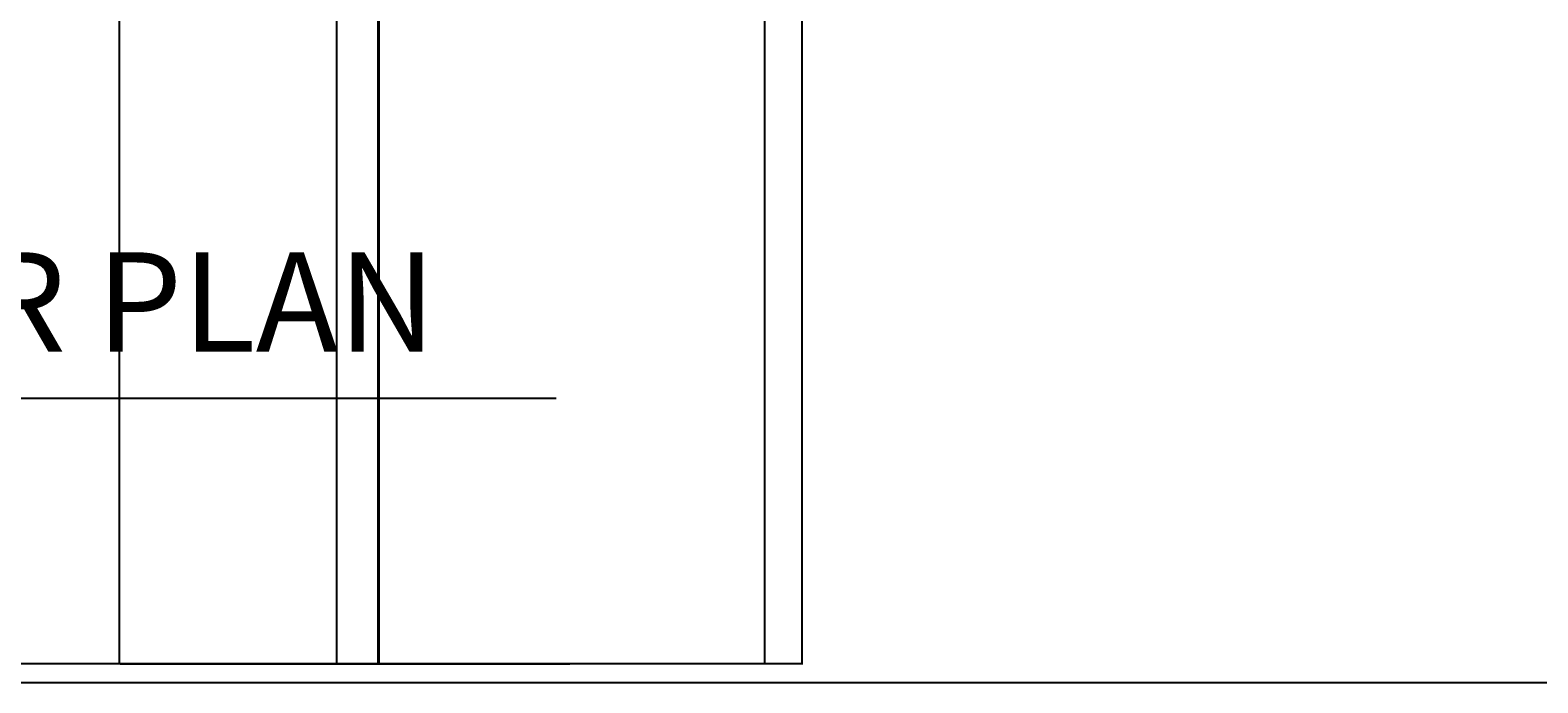
# Model space of a CAD drawing. Units: inches. Extents: x 1770 to 2988, y 1161 to 3221.
# Tile 2 of 44: x 2439 to 2804, y 1161 to 1319. Entities that reach past the tile are written whole.
import ezdxf

# ---------------------------------------------------------------- set-up
doc = ezdxf.new("R2010")
doc.units = ezdxf.units.IN
for name, color, linetype, lineweight in [('A-ANNO-DIMS', 2, 'Continuous', 18), ('A-ANNO-TEXT', 7, 'Continuous', 25), ('A-ANNO-TTLB', 7, 'Continuous', 25)]:
    doc.layers.add(name, color=color, linetype=linetype, lineweight=lineweight)
doc.styles.get("Standard").update_dxf_attribs({"font": 'arial.ttf'})
doc.dimstyles.get("Standard").update_dxf_attribs({"dimtxt": 0.18, "dimasz": 0.18, "dimexe": 0.18, "dimexo": 0.0625, "dimgap": 0.09, "dimtad": 0, "dimtih": 1, "dimtoh": 1, "dimdec": 4, "dimzin": 0, "dimdsep": 46, "dimtxsty": 'Standard', "dimcen": 0.09, "dimadec": 0, "dimazin": 0, "dimtfac": 1, "dimtdec": 4, "dimtofl": 0, "dimtmove": 0, "dimatfit": 3, "dimfxl": 1, "dimtolj": 1, "dimtzin": 0, "dimarcsym": 0})

# ---------------------------------------------------------------- blocks, each defined once
blk = doc.blocks.new('*D60')
at = {"layer": 'A-ANNO-DIMS', "color": 0, "lineweight": -2, "transparency": 16777216}
for p, q in [((2151.7, 1610.14), (2151.7, 1165.57)), ((2625.7, 1610.14), (2625.7, 1165.57)), ((2151.88, 1165.75), (2388.4, 1165.75)), ((2625.52, 1165.75), (2388.99, 1165.75))]:
    blk.add_line(p, q, dxfattribs=at)
at = {"layer": 'A-ANNO-DIMS', "color": 0, "transparency": 16777216}
for points in [[(2151.88, 1165.78), (2151.88, 1165.72), (2151.7, 1165.75)], [(2625.52, 1165.78), (2625.52, 1165.72), (2625.7, 1165.75)]]:
    blk.add_solid(points, dxfattribs=at)
at = {"layer": 'Defpoints', "color": 0, "transparency": 16777216}
for p in [(2151.7, 1610.2), (2625.7, 1610.2), (2625.7, 1165.75)]:
    blk.add_point(p, dxfattribs=at)
at = {"layer": 'A-ANNO-DIMS', "color": 0, "transparency": 16777216, "insert": (2388.7, 1165.75), "char_height": 0.18, "attachment_point": 5}
blk.add_mtext('\\A1;474', dxfattribs=at)
blk = doc.blocks.new('*D74')
at = {"layer": 'A-ANNO-DIMS', "color": 0, "lineweight": -2, "transparency": 16777216}
for p, q in [((2523.42, 2097.48), (2523.42, 1165.57)), ((2616.7, 2097.48), (2616.7, 1165.57)), ((2523.6, 1165.75), (2569.66, 1165.75)), ((2616.52, 1165.75), (2570.45, 1165.75))]:
    blk.add_line(p, q, dxfattribs=at)
at = {"layer": 'A-ANNO-DIMS', "color": 0, "transparency": 16777216}
for points in [[(2523.6, 1165.78), (2523.6, 1165.72), (2523.42, 1165.75)], [(2616.52, 1165.78), (2616.52, 1165.72), (2616.7, 1165.75)]]:
    blk.add_solid(points, dxfattribs=at)
at = {"layer": 'Defpoints', "color": 0, "transparency": 16777216}
for p in [(2523.42, 2097.54), (2616.7, 2097.54), (2616.7, 1165.75)]:
    blk.add_point(p, dxfattribs=at)
at = {"layer": 'A-ANNO-DIMS', "color": 0, "transparency": 16777216, "insert": (2570.06, 1165.75), "char_height": 0.18, "attachment_point": 5}
blk.add_mtext('\\A1;93.28', dxfattribs=at)
blk = doc.blocks.new('*D77')
at = {"layer": 'A-ANNO-DIMS', "color": 0, "lineweight": -2, "transparency": 16777216}
for p, q in [((2460.7, 1710.64), (2460.7, 1165.57)), ((2616.7, 1710.64), (2616.7, 1165.57)), ((2460.88, 1165.75), (2538.42, 1165.75)), ((2616.52, 1165.75), (2538.98, 1165.75))]:
    blk.add_line(p, q, dxfattribs=at)
at = {"layer": 'A-ANNO-DIMS', "color": 0, "transparency": 16777216}
for points in [[(2460.88, 1165.78), (2460.88, 1165.72), (2460.7, 1165.75)], [(2616.52, 1165.78), (2616.52, 1165.72), (2616.7, 1165.75)]]:
    blk.add_solid(points, dxfattribs=at)
at = {"layer": 'Defpoints', "color": 0, "transparency": 16777216}
for p in [(2460.7, 1710.7), (2616.7, 1710.7), (2616.7, 1165.75)]:
    blk.add_point(p, dxfattribs=at)
at = {"layer": 'A-ANNO-DIMS', "color": 0, "transparency": 16777216, "insert": (2538.7, 1165.75), "char_height": 0.18, "attachment_point": 5}
blk.add_mtext('\\A1;156', dxfattribs=at)
blk = doc.blocks.new('*D85')
at = {"layer": 'A-ANNO-DIMS', "color": 0, "lineweight": -2, "transparency": 16777216}
for p, q in [((2513.2, 1773.14), (2513.2, 1165.57)), ((2523.2, 1773.14), (2523.2, 1165.57)), ((2513.38, 1165.75), (2517.99, 1165.75)), ((2523.02, 1165.75), (2518.41, 1165.75))]:
    blk.add_line(p, q, dxfattribs=at)
at = {"layer": 'A-ANNO-DIMS', "color": 0, "transparency": 16777216}
for points in [[(2513.38, 1165.78), (2513.38, 1165.72), (2513.2, 1165.75)], [(2523.02, 1165.78), (2523.02, 1165.72), (2523.2, 1165.75)]]:
    blk.add_solid(points, dxfattribs=at)
at = {"layer": 'Defpoints', "color": 0, "transparency": 16777216}
for p in [(2513.2, 1773.2), (2523.2, 1773.2), (2523.2, 1165.75)]:
    blk.add_point(p, dxfattribs=at)
at = {"layer": 'A-ANNO-DIMS', "color": 0, "transparency": 16777216, "insert": (2518.2, 1165.75), "char_height": 0.18, "attachment_point": 5}
blk.add_mtext('\\A1;10', dxfattribs=at)

msp = doc.modelspace()

# ---------------------------------------------------------------- linework, layer by layer
at = {"layer": 'A-ANNO-TEXT'}
msp.add_line((2198.6214, 1230.002), (2566.3223, 1230.002), dxfattribs=at)
at = {"layer": 'A-ANNO-TTLB'}
msp.add_lwpolyline([(1769.9155, 3221.2788), (2987.7567, 3221.2788), (2987.7567, 1161.1516), (1769.9155, 1161.1516)], close=True, dxfattribs=at)

# ---------------------------------------------------------------- texts
at = {"layer": 'A-ANNO-TEXT', "insert": (2197.8268, 1265.2621), "char_height": 24, "attachment_point": 1}
msp.add_mtext_dynamic_manual_height_columns('GROUND FLOOR PLAN', width=505.43924, gutter_width=12.5, heights=[0], dxfattribs=at)

# ---------------------------------------------------------------- dimensions: what is measured, and where the dimension line sits
at = {"layer": 'A-ANNO-DIMS'}
for base, p1, p2, override, picture, middle in [((2616.696, 1165.752), (2523.4179, 2097.5443), (2616.696, 2097.5443), {"dimdec": 2, "dimlfac": 1, "dimrnd": 0, "dimzin": 0, "dimdsep": 46, "dimlunit": 2}, '*D74', (2570.0569, 1165.752)), ((2523.196, 1165.752), (2513.196, 1773.2021), (2523.196, 1773.2021), {"dimdec": 0, "dimlfac": 1, "dimrnd": 0, "dimzin": 0, "dimdsep": 46, "dimlunit": 2}, '*D85', (2518.196, 1165.752)), ((2616.696, 1165.752), (2460.696, 1710.7021), (2616.696, 1710.7021), {"dimdec": 0, "dimlfac": 1, "dimrnd": 0, "dimzin": 0, "dimdsep": 46, "dimlunit": 2}, '*D77', (2538.696, 1165.752)), ((2625.696, 1165.752), (2151.696, 1610.2021), (2625.696, 1610.2021), {"dimdec": 0, "dimlfac": 1, "dimrnd": 0, "dimzin": 0, "dimdsep": 46, "dimlunit": 2}, '*D60', (2388.696, 1165.752))]:
    dim = msp.add_linear_dim(base=base, p1=p1, p2=p2, dimstyle='Standard', override=override, dxfattribs=at)
    dim.commit()
    dim.dimension.update_dxf_attribs({"geometry": picture, "text_midpoint": middle})

doc.saveas('drawing.dxf')
